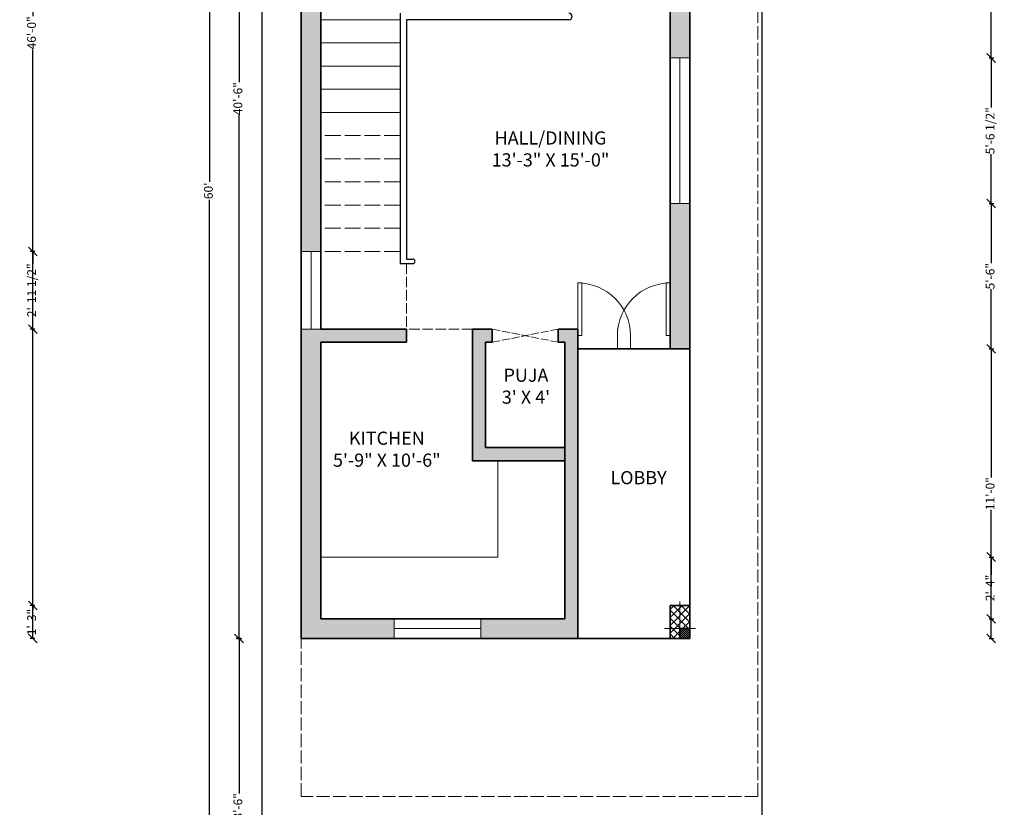
# Model space of a CAD drawing. Units: inches. Extents: x 2349 to 2798, y 397 to 1271.
# Tile 2 of 3: x 2349 to 2798, y 584 to 943. Entities that reach past the tile are written whole.
import ezdxf

# ---------------------------------------------------------------- set-up
doc = ezdxf.new("R2010")
doc.units = ezdxf.units.IN
doc.linetypes.add('ACAD_ISO02W100', pattern=[15, 12, -3])
for name, color, linetype, lineweight in [('A-ANNO-DIMS', 2, 'Continuous', 18), ('A-AREA-IDEN', 7, 'Continuous', 18), ('A-COLS', 1, 'Continuous', 35), ('A-COLS-CNTR', 253, 'Continuous', 13), ('A-COLS-PATT', 8, 'Continuous', 13), ('A-DOOR', 4, 'Continuous', 18), ('A-FLOR-FIXT', 30, 'Continuous', 18), ('A-FLOR-HRAL', 132, 'Continuous', 25), ('A-FLOR-OVHD', 253, 'ACAD_ISO02W100', 13), ('A-FLOR-STRS', 8, 'Continuous', 18), ('A-FLOR-STRS-OVHD', 8, 'ACAD_ISO02W100', 13), ('A-GLAZ', 4, 'Continuous', 18), ('A-WALL', 7, 'Continuous', 35), ('A-WALL-OVHD', 8, 'ACAD_ISO02W100', 13), ('A-WALL-PATT', 8, 'Continuous', 13), ('C-PROP', 7, 'Continuous', 25)]:
    doc.layers.add(name, color=color, linetype=linetype, lineweight=lineweight)
doc.styles.get("Standard").update_dxf_attribs({"font": 'arial.ttf'})
doc.dimstyles.new('ISO-25', dxfattribs={"dimtxt": 4, "dimasz": 4, "dimexe": 1.25, "dimexo": 1, "dimtad": 0, "dimdec": 1, "dimlunit": 3, "dimtxsty": 'Standard', "dimblk": 'OBLIQUE', "dimcen": 2.5, "dimclrd": 1, "dimclrt": 3, "dimadec": 0, "dimazin": 0, "dimtfac": 1, "dimtdec": 1, "dimtmove": 0, "dimatfit": 3, "dimfxl": 1, "dimfxlon": 1, "dimarcsym": 0})

# ---------------------------------------------------------------- blocks, each defined once
blk = doc.blocks.new('_Oblique')
at = {"color": 0, "linetype": 'ByBlock', "lineweight": -2}
blk.add_line((-0.5, -0.5), (0.5, 0.5), dxfattribs=at)
blk = doc.blocks.new('*D8')
at = {"layer": 'A-ANNO-DIMS', "color": 0, "lineweight": -2, "transparency": 16777216}
for p, q in [((2450.39, 1152.52), (2448.14, 1152.52)), ((2449.39, 1152.52), (2449.39, 914.09)), ((2449.39, 660.52), (2449.39, 898.94)), ((2448.39, 660.52), (2450.64, 660.52))]:
    blk.add_line(p, q, dxfattribs=at)
at = {"layer": 'Defpoints', "color": 0, "transparency": 16777216}
for p in [(2459.73, 1152.52), (2435.42, 660.52), (2449.39, 660.52)]:
    blk.add_point(p, dxfattribs=at)
at = {"layer": 'A-ANNO-DIMS', "color": 0, "lineweight": -2, "transparency": 16777216, "xscale": 4, "yscale": 4, "zscale": 4}
for p, rotation in [((2449.39, 1152.52), 90), ((2449.39, 660.52), 270)]:
    blk.add_blockref('_Oblique', p, dxfattribs=dict(at, rotation=rotation))
at = {"layer": 'A-ANNO-DIMS', "color": 0, "transparency": 16777216, "insert": (2449.39, 906.52), "char_height": 4, "attachment_point": 5, "rotation": 90}
blk.add_mtext('40\'-6"', dxfattribs=at)
blk = doc.blocks.new('*D9')
at = {"layer": 'A-ANNO-DIMS', "color": 0, "lineweight": -2, "transparency": 16777216}
for p, q in [((2450.39, 660.52), (2448.14, 660.52)), ((2449.39, 660.52), (2449.39, 589.82)), ((2449.39, 504.52), (2449.39, 575.21)), ((2450.39, 504.52), (2448.14, 504.52))]:
    blk.add_line(p, q, dxfattribs=at)
at = {"layer": 'Defpoints', "color": 0, "transparency": 16777216}
for p in [(2459.73, 660.52), (2449.39, 504.52), (2459.73, 504.52)]:
    blk.add_point(p, dxfattribs=at)
at = {"layer": 'A-ANNO-DIMS', "color": 0, "lineweight": -2, "transparency": 16777216, "xscale": 4, "yscale": 4, "zscale": 4}
for p, rotation in [((2449.39, 660.52), 90), ((2449.39, 504.52), 270)]:
    blk.add_blockref('_Oblique', p, dxfattribs=dict(at, rotation=rotation))
at = {"layer": 'A-ANNO-DIMS', "color": 0, "transparency": 16777216, "insert": (2449.39, 582.52), "char_height": 4, "attachment_point": 5, "rotation": 90}
blk.add_mtext('13\'-6"', dxfattribs=at)
blk = doc.blocks.new('*D10')
at = {"layer": 'A-ANNO-DIMS', "color": 0, "lineweight": -2, "transparency": 16777216}
for p, q in [((2436.96, 1224.52), (2434.71, 1224.52)), ((2435.96, 1224.52), (2435.96, 868.55)), ((2435.96, 504.52), (2435.96, 860.49)), ((2436.96, 504.52), (2434.71, 504.52))]:
    blk.add_line(p, q, dxfattribs=at)
at = {"layer": 'Defpoints', "color": 0, "transparency": 16777216}
for p in [(2459.73, 1224.52), (2435.96, 504.52), (2459.73, 504.52)]:
    blk.add_point(p, dxfattribs=at)
at = {"layer": 'A-ANNO-DIMS', "color": 0, "lineweight": -2, "transparency": 16777216, "xscale": 4, "yscale": 4, "zscale": 4}
for p, rotation in [((2435.96, 1224.52), 90), ((2435.96, 504.52), 270)]:
    blk.add_blockref('_Oblique', p, dxfattribs=dict(at, rotation=rotation))
at = {"layer": 'A-ANNO-DIMS', "color": 0, "transparency": 16777216, "insert": (2435.96, 864.52), "char_height": 4, "attachment_point": 5, "rotation": 90}
blk.add_mtext("60'", dxfattribs=at)
blk = doc.blocks.new('*U16')
for p, q in [((0, 0), (0, -6)), ((24, 0), (24, -6))]:
    blk.add_line(p, q)
blk.add_lwpolyline([(0, 0), (0, 24), (1.75, 24), (1.75, 0)], close=True)
blk.add_arc((0, 0), 24, 0, 90)
blk = doc.blocks.new('*U15')
for p, q in [((-24, 0), (-24, -6)), ((0, 0), (0, -6))]:
    blk.add_line(p, q)
blk.add_lwpolyline([(0, 0), (0, 24), (-1.75, 24), (-1.75, 0)], close=True)
blk.add_arc((0, 0), 24, 90, 180)
blk = doc.blocks.new('*D19')
at = {"layer": 'A-ANNO-DIMS', "color": 0, "lineweight": -2, "transparency": 16777216}
for p, q in [((2356.46, 1212.52), (2354.21, 1212.52)), ((2356.46, 660.52), (2354.21, 660.52))]:
    blk.add_line(p, q, dxfattribs=at)
at = {"layer": 'A-ANNO-DIMS', "color": 1, "lineweight": -2, "transparency": 16777216}
for p, q in [((2355.46, 1212.52), (2355.46, 944.09)), ((2355.46, 660.52), (2355.46, 928.94))]:
    blk.add_line(p, q, dxfattribs=at)
at = {"layer": 'Defpoints', "color": 0, "transparency": 16777216}
for p in [(2355.46, 1212.52), (2477.73, 1212.52), (2477.73, 660.52)]:
    blk.add_point(p, dxfattribs=at)
at = {"layer": 'A-ANNO-DIMS', "color": 1, "lineweight": -2, "transparency": 16777216, "xscale": 4, "yscale": 4, "zscale": 4}
for p, rotation in [((2355.46, 1212.52), 90), ((2355.46, 660.52), 270)]:
    blk.add_blockref('_Oblique', p, dxfattribs=dict(at, rotation=rotation))
at = {"layer": 'A-ANNO-DIMS', "color": 3, "transparency": 16777216, "insert": (2355.46, 936.52), "char_height": 4, "attachment_point": 5, "rotation": 90}
blk.add_mtext('46\'-0"', dxfattribs=at)
blk = doc.blocks.new('*D20')
at = {"layer": 'A-ANNO-DIMS', "color": 0, "lineweight": -2, "transparency": 16777216}
for p, q in [((2790.99, 792.52), (2793.24, 792.52)), ((2790.99, 660.52), (2793.24, 660.52))]:
    blk.add_line(p, q, dxfattribs=at)
at = {"layer": 'A-ANNO-DIMS', "color": 1, "lineweight": -2, "transparency": 16777216}
for p, q in [((2791.99, 792.52), (2791.99, 733.82)), ((2791.99, 660.52), (2791.99, 719.21))]:
    blk.add_line(p, q, dxfattribs=at)
at = {"layer": 'Defpoints', "color": 0, "transparency": 16777216}
for p in [(2654.73, 792.52), (2791.99, 792.52), (2654.73, 660.52)]:
    blk.add_point(p, dxfattribs=at)
at = {"layer": 'A-ANNO-DIMS', "color": 1, "lineweight": -2, "transparency": 16777216, "xscale": 4, "yscale": 4, "zscale": 4}
for p, rotation in [((2791.99, 792.52), 90), ((2791.99, 660.52), 270)]:
    blk.add_blockref('_Oblique', p, dxfattribs=dict(at, rotation=rotation))
at = {"layer": 'A-ANNO-DIMS', "color": 3, "transparency": 16777216, "insert": (2791.99, 726.52), "char_height": 4, "attachment_point": 5, "rotation": 90}
blk.add_mtext('11\'-0"', dxfattribs=at)
blk = doc.blocks.new('*D21')
at = {"layer": 'A-ANNO-DIMS', "color": 0, "lineweight": -2, "transparency": 16777216}
for p, q in [((2790.99, 858.74), (2793.24, 858.74)), ((2790.99, 792.52), (2793.24, 792.52))]:
    blk.add_line(p, q, dxfattribs=at)
at = {"layer": 'A-ANNO-DIMS', "color": 1, "lineweight": -2, "transparency": 16777216}
for p, q in [((2791.99, 858.74), (2791.99, 831.57)), ((2791.99, 792.52), (2791.99, 819.69))]:
    blk.add_line(p, q, dxfattribs=at)
at = {"layer": 'Defpoints', "color": 0, "transparency": 16777216}
for p in [(2654.73, 858.74), (2791.99, 858.74), (2654.73, 792.52)]:
    blk.add_point(p, dxfattribs=at)
at = {"layer": 'A-ANNO-DIMS', "color": 1, "lineweight": -2, "transparency": 16777216, "xscale": 4, "yscale": 4, "zscale": 4}
for p, rotation in [((2791.99, 858.74), 90), ((2791.99, 792.52), 270)]:
    blk.add_blockref('_Oblique', p, dxfattribs=dict(at, rotation=rotation))
at = {"layer": 'A-ANNO-DIMS', "color": 3, "transparency": 16777216, "insert": (2791.99, 825.63), "char_height": 4, "attachment_point": 5, "rotation": 90}
blk.add_mtext('5\'-6"', dxfattribs=at)
blk = doc.blocks.new('*D22')
at = {"layer": 'A-ANNO-DIMS', "color": 0, "lineweight": -2, "transparency": 16777216}
for p, q in [((2790.99, 925.07), (2793.24, 925.07)), ((2790.99, 858.74), (2793.24, 858.74))]:
    blk.add_line(p, q, dxfattribs=at)
at = {"layer": 'A-ANNO-DIMS', "color": 1, "lineweight": -2, "transparency": 16777216}
for p, q in [((2791.99, 925.07), (2791.99, 902.51)), ((2791.99, 858.74), (2791.99, 881.3))]:
    blk.add_line(p, q, dxfattribs=at)
at = {"layer": 'Defpoints', "color": 0, "transparency": 16777216}
for p in [(2654.73, 925.07), (2791.99, 925.07), (2654.73, 858.74)]:
    blk.add_point(p, dxfattribs=at)
at = {"layer": 'A-ANNO-DIMS', "color": 1, "lineweight": -2, "transparency": 16777216, "xscale": 4, "yscale": 4, "zscale": 4}
for p, rotation in [((2791.99, 925.07), 90), ((2791.99, 858.74), 270)]:
    blk.add_blockref('_Oblique', p, dxfattribs=dict(at, rotation=rotation))
at = {"layer": 'A-ANNO-DIMS', "color": 3, "transparency": 16777216, "insert": (2791.99, 891.9), "char_height": 4, "attachment_point": 5, "rotation": 90}
blk.add_mtext('5\'-6 1/2"', dxfattribs=at)
blk = doc.blocks.new('*D23')
at = {"layer": 'A-ANNO-DIMS', "color": 0, "lineweight": -2, "transparency": 16777216}
for p, q in [((2790.99, 1010.67), (2793.24, 1010.67)), ((2790.99, 925.07), (2793.24, 925.07))]:
    blk.add_line(p, q, dxfattribs=at)
at = {"layer": 'A-ANNO-DIMS', "color": 1, "lineweight": -2, "transparency": 16777216}
for p, q in [((2791.99, 1010.67), (2791.99, 978.45)), ((2791.99, 925.07), (2791.99, 957.28))]:
    blk.add_line(p, q, dxfattribs=at)
at = {"layer": 'Defpoints', "color": 0, "transparency": 16777216}
for p in [(2654.73, 1010.67), (2791.99, 1010.67), (2654.73, 925.07)]:
    blk.add_point(p, dxfattribs=at)
at = {"layer": 'A-ANNO-DIMS', "color": 1, "lineweight": -2, "transparency": 16777216, "xscale": 4, "yscale": 4, "zscale": 4}
for p, rotation in [((2791.99, 1010.67), 90), ((2791.99, 925.07), 270)]:
    blk.add_blockref('_Oblique', p, dxfattribs=dict(at, rotation=rotation))
at = {"layer": 'A-ANNO-DIMS', "color": 3, "transparency": 16777216, "insert": (2791.99, 967.87), "char_height": 4, "attachment_point": 5, "rotation": 90}
blk.add_mtext('7\'-1 1/2"', dxfattribs=at)
blk = doc.blocks.new('*D28')
at = {"layer": 'A-ANNO-DIMS', "color": 0, "lineweight": -2, "transparency": 16777216}
for p, q in [((2603.73, 403.67), (2603.73, 401.42)), ((2654.73, 403.67), (2654.73, 401.42))]:
    blk.add_line(p, q, dxfattribs=at)
at = {"layer": 'A-ANNO-DIMS', "color": 1, "lineweight": -2, "transparency": 16777216}
for p, q in [((2603.73, 402.67), (2623.21, 402.67)), ((2654.73, 402.67), (2635.25, 402.67))]:
    blk.add_line(p, q, dxfattribs=at)
at = {"layer": 'Defpoints', "color": 0, "transparency": 16777216}
for p in [(2603.73, 660.52), (2654.73, 660.52), (2654.73, 402.67)]:
    blk.add_point(p, dxfattribs=at)
at = {"layer": 'A-ANNO-DIMS', "color": 1, "lineweight": -2, "transparency": 16777216, "xscale": 4, "yscale": 4, "zscale": 4, "rotation": 180}
blk.add_blockref('_Oblique', (2603.73, 402.67), dxfattribs=at)
at = {"layer": 'A-ANNO-DIMS', "color": 1, "lineweight": -2, "transparency": 16777216, "xscale": 4, "yscale": 4, "zscale": 4}
blk.add_blockref('_Oblique', (2654.73, 402.67), dxfattribs=at)
at = {"layer": 'A-ANNO-DIMS', "color": 3, "transparency": 16777216, "insert": (2629.23, 402.67), "char_height": 4, "attachment_point": 5}
blk.add_mtext('4\'-3"', dxfattribs=at)
blk = doc.blocks.new('*D29')
at = {"layer": 'A-ANNO-DIMS', "color": 0, "lineweight": -2, "transparency": 16777216}
for p, q in [((2477.73, 403.67), (2477.73, 401.42)), ((2520.04, 403.67), (2520.04, 401.42))]:
    blk.add_line(p, q, dxfattribs=at)
at = {"layer": 'A-ANNO-DIMS', "color": 1, "lineweight": -2, "transparency": 16777216}
for p, q in [((2477.73, 402.67), (2488.28, 402.67)), ((2520.04, 402.67), (2509.48, 402.67))]:
    blk.add_line(p, q, dxfattribs=at)
at = {"layer": 'Defpoints', "color": 0, "transparency": 16777216}
for p in [(2477.73, 660.52), (2520.04, 660.52), (2520.04, 402.67)]:
    blk.add_point(p, dxfattribs=at)
at = {"layer": 'A-ANNO-DIMS', "color": 1, "lineweight": -2, "transparency": 16777216, "xscale": 4, "yscale": 4, "zscale": 4, "rotation": 180}
blk.add_blockref('_Oblique', (2477.73, 402.67), dxfattribs=at)
at = {"layer": 'A-ANNO-DIMS', "color": 1, "lineweight": -2, "transparency": 16777216, "xscale": 4, "yscale": 4, "zscale": 4}
blk.add_blockref('_Oblique', (2520.04, 402.67), dxfattribs=at)
at = {"layer": 'A-ANNO-DIMS', "color": 3, "transparency": 16777216, "insert": (2498.88, 402.67), "char_height": 4, "attachment_point": 5}
blk.add_mtext('3\'-6 1/2"', dxfattribs=at)
blk = doc.blocks.new('*D30')
at = {"layer": 'A-ANNO-DIMS', "color": 0, "lineweight": -2, "transparency": 16777216}
for p, q in [((2520.04, 403.67), (2520.04, 401.42)), ((2559.59, 403.67), (2559.59, 401.42))]:
    blk.add_line(p, q, dxfattribs=at)
at = {"layer": 'A-ANNO-DIMS', "color": 1, "lineweight": -2, "transparency": 16777216}
for p, q in [((2520.04, 402.67), (2529.21, 402.67)), ((2559.59, 402.67), (2550.42, 402.67))]:
    blk.add_line(p, q, dxfattribs=at)
at = {"layer": 'Defpoints', "color": 0, "transparency": 16777216}
for p in [(2520.04, 660.52), (2559.59, 660.52), (2559.59, 402.67)]:
    blk.add_point(p, dxfattribs=at)
at = {"layer": 'A-ANNO-DIMS', "color": 1, "lineweight": -2, "transparency": 16777216, "xscale": 4, "yscale": 4, "zscale": 4, "rotation": 180}
blk.add_blockref('_Oblique', (2520.04, 402.67), dxfattribs=at)
at = {"layer": 'A-ANNO-DIMS', "color": 1, "lineweight": -2, "transparency": 16777216, "xscale": 4, "yscale": 4, "zscale": 4}
blk.add_blockref('_Oblique', (2559.59, 402.67), dxfattribs=at)
at = {"layer": 'A-ANNO-DIMS', "color": 3, "transparency": 16777216, "insert": (2539.81, 402.67), "char_height": 4, "attachment_point": 5}
blk.add_mtext('3\'-3 1/2"', dxfattribs=at)
blk = doc.blocks.new('*D31')
at = {"layer": 'A-ANNO-DIMS', "color": 0, "lineweight": -2, "transparency": 16777216}
for p, q in [((2603.73, 403.67), (2603.73, 401.42)), ((2645.73, 403.67), (2645.73, 401.42))]:
    blk.add_line(p, q, dxfattribs=at)
at = {"layer": 'A-ANNO-DIMS', "color": 1, "lineweight": -2, "transparency": 16777216}
for p, q in [((2603.73, 402.67), (2618.79, 402.67)), ((2645.73, 402.67), (2630.67, 402.67))]:
    blk.add_line(p, q, dxfattribs=at)
at = {"layer": 'Defpoints', "color": 0, "transparency": 16777216}
for p in [(2603.73, 792.52), (2645.73, 792.52), (2645.73, 402.67)]:
    blk.add_point(p, dxfattribs=at)
at = {"layer": 'A-ANNO-DIMS', "color": 1, "lineweight": -2, "transparency": 16777216, "xscale": 4, "yscale": 4, "zscale": 4, "rotation": 180}
blk.add_blockref('_Oblique', (2603.73, 402.67), dxfattribs=at)
at = {"layer": 'A-ANNO-DIMS', "color": 1, "lineweight": -2, "transparency": 16777216, "xscale": 4, "yscale": 4, "zscale": 4}
blk.add_blockref('_Oblique', (2645.73, 402.67), dxfattribs=at)
at = {"layer": 'A-ANNO-DIMS', "color": 3, "transparency": 16777216, "insert": (2624.73, 402.67), "char_height": 4, "attachment_point": 5}
blk.add_mtext('3\'-6"', dxfattribs=at)
blk = doc.blocks.new('*D32')
at = {"layer": 'A-ANNO-DIMS', "color": 0, "lineweight": -2, "transparency": 16777216}
for p, q in [((2606.73, 403.67), (2606.73, 401.42)), ((2642.73, 403.67), (2642.73, 401.42))]:
    blk.add_line(p, q, dxfattribs=at)
at = {"layer": 'A-ANNO-DIMS', "color": 1, "lineweight": -2, "transparency": 16777216}
for p, q in [((2606.73, 402.67), (2618.79, 402.67)), ((2642.73, 402.67), (2630.67, 402.67))]:
    blk.add_line(p, q, dxfattribs=at)
at = {"layer": 'Defpoints', "color": 0, "transparency": 16777216}
for p in [(2606.73, 981.52), (2642.73, 981.52), (2642.73, 402.67)]:
    blk.add_point(p, dxfattribs=at)
at = {"layer": 'A-ANNO-DIMS', "color": 1, "lineweight": -2, "transparency": 16777216, "xscale": 4, "yscale": 4, "zscale": 4, "rotation": 180}
blk.add_blockref('_Oblique', (2606.73, 402.67), dxfattribs=at)
at = {"layer": 'A-ANNO-DIMS', "color": 1, "lineweight": -2, "transparency": 16777216, "xscale": 4, "yscale": 4, "zscale": 4}
blk.add_blockref('_Oblique', (2642.73, 402.67), dxfattribs=at)
at = {"layer": 'A-ANNO-DIMS', "color": 3, "transparency": 16777216, "insert": (2624.73, 402.67), "char_height": 4, "attachment_point": 5}
blk.add_mtext('3\'-0"', dxfattribs=at)
blk = doc.blocks.new('*D33')
at = {"layer": 'A-ANNO-DIMS', "color": 0, "lineweight": -2, "transparency": 16777216}
for p, q in [((2556.73, 403.67), (2556.73, 401.42)), ((2588.73, 403.67), (2588.73, 401.42))]:
    blk.add_line(p, q, dxfattribs=at)
at = {"layer": 'A-ANNO-DIMS', "color": 1, "lineweight": -2, "transparency": 16777216}
for p, q in [((2556.73, 402.67), (2566.76, 402.67)), ((2588.73, 402.67), (2578.71, 402.67))]:
    blk.add_line(p, q, dxfattribs=at)
at = {"layer": 'Defpoints', "color": 0, "transparency": 16777216}
for p in [(2556.73, 1143.52), (2588.73, 1143.52), (2588.73, 402.67)]:
    blk.add_point(p, dxfattribs=at)
at = {"layer": 'A-ANNO-DIMS', "color": 1, "lineweight": -2, "transparency": 16777216, "xscale": 4, "yscale": 4, "zscale": 4, "rotation": 180}
blk.add_blockref('_Oblique', (2556.73, 402.67), dxfattribs=at)
at = {"layer": 'A-ANNO-DIMS', "color": 1, "lineweight": -2, "transparency": 16777216, "xscale": 4, "yscale": 4, "zscale": 4}
blk.add_blockref('_Oblique', (2588.73, 402.67), dxfattribs=at)
at = {"layer": 'A-ANNO-DIMS', "color": 3, "transparency": 16777216, "insert": (2572.73, 402.67), "char_height": 4, "attachment_point": 5}
blk.add_mtext('2\'-8"', dxfattribs=at)
blk = doc.blocks.new('*D38')
at = {"layer": 'A-ANNO-DIMS', "color": 0, "lineweight": -2, "transparency": 16777216}
for p, q in [((2356.46, 836.92), (2354.21, 836.92)), ((2356.46, 801.52), (2354.21, 801.52))]:
    blk.add_line(p, q, dxfattribs=at)
at = {"layer": 'A-ANNO-DIMS', "color": 1, "lineweight": -2, "transparency": 16777216}
for p, q in [((2355.46, 836.92), (2355.46, 831.41)), ((2355.46, 801.52), (2355.46, 807.03))]:
    blk.add_line(p, q, dxfattribs=at)
at = {"layer": 'Defpoints', "color": 0, "transparency": 16777216}
for p in [(2355.46, 836.92), (2477.73, 836.92), (2477.73, 801.52)]:
    blk.add_point(p, dxfattribs=at)
at = {"layer": 'A-ANNO-DIMS', "color": 1, "lineweight": -2, "transparency": 16777216, "xscale": 4, "yscale": 4, "zscale": 4}
for p, rotation in [((2355.46, 836.92), 90), ((2355.46, 801.52), 270)]:
    blk.add_blockref('_Oblique', p, dxfattribs=dict(at, rotation=rotation))
at = {"layer": 'A-ANNO-DIMS', "color": 3, "transparency": 16777216, "insert": (2355.46, 819.22), "char_height": 4, "attachment_point": 5, "rotation": 90}
blk.add_mtext('2\'-11 1/2"', dxfattribs=at)
blk = doc.blocks.new('*D39')
at = {"layer": 'A-ANNO-DIMS', "color": 0, "lineweight": -2, "transparency": 16777216}
for p, q in [((2486.73, 403.67), (2486.73, 401.42)), ((2522.73, 403.67), (2522.73, 401.42))]:
    blk.add_line(p, q, dxfattribs=at)
at = {"layer": 'A-ANNO-DIMS', "color": 1, "lineweight": -2, "transparency": 16777216}
for p, q in [((2486.73, 402.67), (2498.79, 402.67)), ((2522.73, 402.67), (2510.67, 402.67))]:
    blk.add_line(p, q, dxfattribs=at)
at = {"layer": 'Defpoints', "color": 0, "transparency": 16777216}
for p in [(2486.73, 836.92), (2522.73, 836.92), (2522.73, 402.67)]:
    blk.add_point(p, dxfattribs=at)
at = {"layer": 'A-ANNO-DIMS', "color": 1, "lineweight": -2, "transparency": 16777216, "xscale": 4, "yscale": 4, "zscale": 4, "rotation": 180}
blk.add_blockref('_Oblique', (2486.73, 402.67), dxfattribs=at)
at = {"layer": 'A-ANNO-DIMS', "color": 1, "lineweight": -2, "transparency": 16777216, "xscale": 4, "yscale": 4, "zscale": 4}
blk.add_blockref('_Oblique', (2522.73, 402.67), dxfattribs=at)
at = {"layer": 'A-ANNO-DIMS', "color": 3, "transparency": 16777216, "insert": (2504.73, 402.67), "char_height": 4, "attachment_point": 5}
blk.add_mtext('3\'-0"', dxfattribs=at)
blk = doc.blocks.new('*D40')
at = {"layer": 'A-ANNO-DIMS', "color": 0, "lineweight": -2, "transparency": 16777216}
for p, q in [((2525.73, 403.67), (2525.73, 401.42)), ((2555.73, 403.67), (2555.73, 401.42))]:
    blk.add_line(p, q, dxfattribs=at)
at = {"layer": 'A-ANNO-DIMS', "color": 1, "lineweight": -2, "transparency": 16777216}
for p, q in [((2525.73, 402.67), (2534.76, 402.67)), ((2555.73, 402.67), (2546.71, 402.67))]:
    blk.add_line(p, q, dxfattribs=at)
at = {"layer": 'Defpoints', "color": 0, "transparency": 16777216}
for p in [(2555.73, 801.52), (2525.73, 795.52), (2555.73, 402.67)]:
    blk.add_point(p, dxfattribs=at)
at = {"layer": 'A-ANNO-DIMS', "color": 1, "lineweight": -2, "transparency": 16777216, "xscale": 4, "yscale": 4, "zscale": 4, "rotation": 180}
blk.add_blockref('_Oblique', (2525.73, 402.67), dxfattribs=at)
at = {"layer": 'A-ANNO-DIMS', "color": 1, "lineweight": -2, "transparency": 16777216, "xscale": 4, "yscale": 4, "zscale": 4}
blk.add_blockref('_Oblique', (2555.73, 402.67), dxfattribs=at)
at = {"layer": 'A-ANNO-DIMS', "color": 3, "transparency": 16777216, "insert": (2540.73, 402.67), "char_height": 4, "attachment_point": 5}
blk.add_mtext('2\'-6"', dxfattribs=at)
blk = doc.blocks.new('*D41')
at = {"layer": 'A-ANNO-DIMS', "color": 0, "lineweight": -2, "transparency": 16777216}
for p, q in [((2564.73, 1264.12), (2564.73, 1266.37)), ((2594.73, 1264.12), (2594.73, 1266.37))]:
    blk.add_line(p, q, dxfattribs=at)
at = {"layer": 'A-ANNO-DIMS', "color": 1, "lineweight": -2, "transparency": 16777216}
for p, q in [((2564.73, 1265.12), (2573.76, 1265.12)), ((2594.73, 1265.12), (2585.71, 1265.12))]:
    blk.add_line(p, q, dxfattribs=at)
at = {"layer": 'Defpoints', "color": 0, "transparency": 16777216}
for p in [(2594.73, 1265.12), (2564.73, 801.52), (2594.73, 801.52)]:
    blk.add_point(p, dxfattribs=at)
at = {"layer": 'A-ANNO-DIMS', "color": 1, "lineweight": -2, "transparency": 16777216, "xscale": 4, "yscale": 4, "zscale": 4, "rotation": 180}
blk.add_blockref('_Oblique', (2564.73, 1265.12), dxfattribs=at)
at = {"layer": 'A-ANNO-DIMS', "color": 1, "lineweight": -2, "transparency": 16777216, "xscale": 4, "yscale": 4, "zscale": 4}
blk.add_blockref('_Oblique', (2594.73, 1265.12), dxfattribs=at)
at = {"layer": 'A-ANNO-DIMS', "color": 3, "transparency": 16777216, "insert": (2579.73, 1265.12), "char_height": 4, "attachment_point": 5}
blk.add_mtext('2\'-6"', dxfattribs=at)
blk = doc.blocks.new('*D42')
at = {"layer": 'A-ANNO-DIMS', "color": 0, "lineweight": -2, "transparency": 16777216}
for p, q in [((2567.33, 1264.12), (2567.33, 1266.37)), ((2597.73, 1264.12), (2597.73, 1266.37))]:
    blk.add_line(p, q, dxfattribs=at)
at = {"layer": 'A-ANNO-DIMS', "color": 1, "lineweight": -2, "transparency": 16777216}
for p, q in [((2567.33, 1265.12), (2571.89, 1265.12)), ((2597.73, 1265.12), (2593.16, 1265.12))]:
    blk.add_line(p, q, dxfattribs=at)
at = {"layer": 'Defpoints', "color": 0, "transparency": 16777216}
for p in [(2567.33, 1265.12), (2567.33, 697.63), (2597.73, 669.52)]:
    blk.add_point(p, dxfattribs=at)
at = {"layer": 'A-ANNO-DIMS', "color": 1, "lineweight": -2, "transparency": 16777216, "xscale": 4, "yscale": 4, "zscale": 4, "rotation": 180}
blk.add_blockref('_Oblique', (2567.33, 1265.12), dxfattribs=at)
at = {"layer": 'A-ANNO-DIMS', "color": 1, "lineweight": -2, "transparency": 16777216, "xscale": 4, "yscale": 4, "zscale": 4}
blk.add_blockref('_Oblique', (2597.73, 1265.12), dxfattribs=at)
at = {"layer": 'A-ANNO-DIMS', "color": 3, "transparency": 16777216, "insert": (2582.53, 1265.12), "char_height": 4, "attachment_point": 5}
blk.add_mtext('2\'-6 1/2"', dxfattribs=at)
blk = doc.blocks.new('*D43')
at = {"layer": 'A-ANNO-DIMS', "color": 0, "lineweight": -2, "transparency": 16777216}
for p, q in [((2790.99, 697.63), (2793.24, 697.63)), ((2790.99, 669.52), (2793.24, 669.52))]:
    blk.add_line(p, q, dxfattribs=at)
at = {"layer": 'A-ANNO-DIMS', "color": 1, "lineweight": -2, "transparency": 16777216}
for p, q in [((2791.99, 697.63), (2791.99, 689.55)), ((2791.99, 669.52), (2791.99, 677.6))]:
    blk.add_line(p, q, dxfattribs=at)
at = {"layer": 'Defpoints', "color": 0, "transparency": 16777216}
for p in [(2486.73, 697.63), (2791.99, 697.63), (2486.73, 669.52)]:
    blk.add_point(p, dxfattribs=at)
at = {"layer": 'A-ANNO-DIMS', "color": 1, "lineweight": -2, "transparency": 16777216, "xscale": 4, "yscale": 4, "zscale": 4}
for p, rotation in [((2791.99, 697.63), 90), ((2791.99, 669.52), 270)]:
    blk.add_blockref('_Oblique', p, dxfattribs=dict(at, rotation=rotation))
at = {"layer": 'A-ANNO-DIMS', "color": 3, "transparency": 16777216, "insert": (2791.99, 683.57), "char_height": 4, "attachment_point": 5, "rotation": 90}
blk.add_mtext('2\'-4"', dxfattribs=at)
blk = doc.blocks.new('*D44')
at = {"layer": 'A-ANNO-DIMS', "color": 0, "lineweight": -2, "transparency": 16777216}
for p, q in [((2645.73, 1264.12), (2645.73, 1266.37)), ((2654.73, 1264.12), (2654.73, 1266.37))]:
    blk.add_line(p, q, dxfattribs=at)
at = {"layer": 'A-ANNO-DIMS', "color": 1, "lineweight": -2, "transparency": 16777216}
for p, q in [((2645.73, 1265.12), (2654.73, 1265.12)), ((2654.73, 1265.12), (2658.73, 1265.12))]:
    blk.add_line(p, q, dxfattribs=at)
at = {"layer": 'Defpoints', "color": 0, "transparency": 16777216}
for p in [(2654.73, 1265.12), (2645.73, 675.52), (2654.73, 675.52)]:
    blk.add_point(p, dxfattribs=at)
at = {"layer": 'A-ANNO-DIMS', "color": 1, "lineweight": -2, "transparency": 16777216, "xscale": 4, "yscale": 4, "zscale": 4, "rotation": 180}
blk.add_blockref('_Oblique', (2645.73, 1265.12), dxfattribs=at)
at = {"layer": 'A-ANNO-DIMS', "color": 1, "lineweight": -2, "transparency": 16777216, "xscale": 4, "yscale": 4, "zscale": 4}
blk.add_blockref('_Oblique', (2654.73, 1265.12), dxfattribs=at)
at = {"layer": 'A-ANNO-DIMS', "color": 3, "transparency": 16777216, "insert": (2664.67, 1265.12), "char_height": 4, "attachment_point": 5}
blk.add_mtext('0\'-9"', dxfattribs=at)
blk = doc.blocks.new('*D45')
at = {"layer": 'A-ANNO-DIMS', "color": 0, "lineweight": -2, "transparency": 16777216}
for p, q in [((2356.46, 675.52), (2354.21, 675.52)), ((2356.46, 660.52), (2354.21, 660.52))]:
    blk.add_line(p, q, dxfattribs=at)
at = {"layer": 'A-ANNO-DIMS', "color": 1, "lineweight": -2, "transparency": 16777216}
for p, q in [((2355.46, 675.52), (2355.46, 673.77)), ((2355.46, 660.52), (2355.46, 662.26))]:
    blk.add_line(p, q, dxfattribs=at)
at = {"layer": 'Defpoints', "color": 0, "transparency": 16777216}
for p in [(2355.46, 675.52), (2645.73, 675.52), (2645.73, 660.52)]:
    blk.add_point(p, dxfattribs=at)
at = {"layer": 'A-ANNO-DIMS', "color": 1, "lineweight": -2, "transparency": 16777216, "xscale": 4, "yscale": 4, "zscale": 4}
for p, rotation in [((2355.46, 675.52), 90), ((2355.46, 660.52), 270)]:
    blk.add_blockref('_Oblique', p, dxfattribs=dict(at, rotation=rotation))
at = {"layer": 'A-ANNO-DIMS', "color": 3, "transparency": 16777216, "insert": (2355.46, 668.02), "char_height": 4, "attachment_point": 5, "rotation": 90}
blk.add_mtext('1\'-3"', dxfattribs=at)
blk = doc.blocks.new('*D46')
at = {"layer": 'A-ANNO-DIMS', "color": 0, "lineweight": -2, "transparency": 16777216}
for p, q in [((2591.73, 403.67), (2591.73, 401.42)), ((2597.73, 403.67), (2597.73, 401.42))]:
    blk.add_line(p, q, dxfattribs=at)
at = {"layer": 'A-ANNO-DIMS', "color": 1, "lineweight": -2, "transparency": 16777216}
for p, q in [((2591.73, 402.67), (2597.73, 402.67)), ((2597.73, 402.67), (2601.73, 402.67))]:
    blk.add_line(p, q, dxfattribs=at)
at = {"layer": 'Defpoints', "color": 0, "transparency": 16777216}
for p in [(2591.73, 1206.52), (2597.73, 1206.52), (2597.73, 402.67)]:
    blk.add_point(p, dxfattribs=at)
at = {"layer": 'A-ANNO-DIMS', "color": 1, "lineweight": -2, "transparency": 16777216, "xscale": 4, "yscale": 4, "zscale": 4, "rotation": 180}
blk.add_blockref('_Oblique', (2591.73, 402.67), dxfattribs=at)
at = {"layer": 'A-ANNO-DIMS', "color": 1, "lineweight": -2, "transparency": 16777216, "xscale": 4, "yscale": 4, "zscale": 4}
blk.add_blockref('_Oblique', (2597.73, 402.67), dxfattribs=at)
at = {"layer": 'A-ANNO-DIMS', "color": 3, "transparency": 16777216, "insert": (2607.67, 402.67), "char_height": 4, "attachment_point": 5}
blk.add_mtext('0\'-6"', dxfattribs=at)
blk = doc.blocks.new('*D47')
at = {"layer": 'A-ANNO-DIMS', "color": 0, "lineweight": -2, "transparency": 16777216}
for p, q in [((2477.73, 403.67), (2477.73, 401.42)), ((2486.73, 403.67), (2486.73, 401.42))]:
    blk.add_line(p, q, dxfattribs=at)
at = {"layer": 'A-ANNO-DIMS', "color": 1, "lineweight": -2, "transparency": 16777216}
for p, q in [((2477.73, 402.67), (2486.73, 402.67)), ((2486.73, 402.67), (2490.73, 402.67))]:
    blk.add_line(p, q, dxfattribs=at)
at = {"layer": 'Defpoints', "color": 0, "transparency": 16777216}
for p in [(2477.73, 1212.52), (2486.73, 1206.52), (2486.73, 402.67)]:
    blk.add_point(p, dxfattribs=at)
at = {"layer": 'A-ANNO-DIMS', "color": 1, "lineweight": -2, "transparency": 16777216, "xscale": 4, "yscale": 4, "zscale": 4, "rotation": 180}
blk.add_blockref('_Oblique', (2477.73, 402.67), dxfattribs=at)
at = {"layer": 'A-ANNO-DIMS', "color": 1, "lineweight": -2, "transparency": 16777216, "xscale": 4, "yscale": 4, "zscale": 4}
blk.add_blockref('_Oblique', (2486.73, 402.67), dxfattribs=at)
at = {"layer": 'A-ANNO-DIMS', "color": 3, "transparency": 16777216, "insert": (2496.67, 402.67), "char_height": 4, "attachment_point": 5}
blk.add_mtext('0\'-9"', dxfattribs=at)
blk = doc.blocks.new('*D48')
at = {"layer": 'A-ANNO-DIMS', "color": 0, "lineweight": -2, "transparency": 16777216}
for p, q in [((2525.73, 403.67), (2525.73, 401.42)), ((2599.63, 403.67), (2599.63, 401.42))]:
    blk.add_line(p, q, dxfattribs=at)
at = {"layer": 'A-ANNO-DIMS', "color": 1, "lineweight": -2, "transparency": 16777216}
for p, q in [((2525.73, 402.67), (2556.73, 402.67)), ((2599.63, 402.67), (2568.63, 402.67))]:
    blk.add_line(p, q, dxfattribs=at)
at = {"layer": 'Defpoints', "color": 0, "transparency": 16777216}
for p in [(2525.73, 942.52), (2599.63, 942.52), (2599.63, 402.67)]:
    blk.add_point(p, dxfattribs=at)
at = {"layer": 'A-ANNO-DIMS', "color": 1, "lineweight": -2, "transparency": 16777216, "xscale": 4, "yscale": 4, "zscale": 4, "rotation": 180}
blk.add_blockref('_Oblique', (2525.73, 402.67), dxfattribs=at)
at = {"layer": 'A-ANNO-DIMS', "color": 1, "lineweight": -2, "transparency": 16777216, "xscale": 4, "yscale": 4, "zscale": 4}
blk.add_blockref('_Oblique', (2599.63, 402.67), dxfattribs=at)
at = {"layer": 'A-ANNO-DIMS', "color": 3, "transparency": 16777216, "insert": (2562.68, 402.67), "char_height": 4, "attachment_point": 5}
blk.add_mtext('6\'-2"', dxfattribs=at)

msp = doc.modelspace()

# ---------------------------------------------------------------- hatches: boundary and pattern name
at = {"layer": 'A-COLS-PATT'}
h = msp.add_hatch(dxfattribs=at)
h.set_pattern_fill('ANSI37', color=256, scale=0.8)
h.paths.add_polyline_path([(2654.73, 675.52), (2645.73, 675.52), (2645.73, 660.52), (2650.23, 660.52), (2650.23, 665.02), (2654.73, 665.02)])
h = msp.add_hatch(dxfattribs=at)
h.set_pattern_fill('ANSI31', color=256, scale=0.2)
h.paths.add_polyline_path([(2654.73, 665.02), (2650.23, 665.02), (2650.23, 660.52), (2654.73, 660.52)])
at = {"layer": 'A-WALL-PATT'}
h = msp.add_hatch(color=256, dxfattribs=at)
h.dxf.hatch_style = 1
h.paths.add_polyline_path([(2616.29, 1212.52), (2561.36, 1212.52), (2561.36, 1206.52), (2591.73, 1206.52), (2591.73, 1152.52), (2588.73, 1152.52), (2588.73, 1143.52), (2645.73, 1143.52), (2645.73, 1070.67), (2654.73, 1070.67), (2654.73, 1155.52), (2645.73, 1155.52), (2645.73, 1152.52), (2597.73, 1152.52), (2597.73, 1206.52), (2616.29, 1206.52)])
h.paths.add_polyline_path([(2654.73, 1212.52), (2637.4, 1212.52), (2637.4, 1206.52), (2645.73, 1206.52), (2645.73, 1183.52), (2654.73, 1183.52)], flags=17)
h.paths.add_polyline_path([(2520.04, 669.52), (2486.73, 669.52), (2486.73, 795.52), (2525.73, 795.52), (2525.73, 801.52), (2486.73, 801.52), (2477.73, 801.52), (2477.73, 660.52), (2520.04, 660.52)])
h.paths.add_polyline_path([(2486.73, 981.52), (2606.73, 981.52), (2606.73, 987.52), (2486.73, 987.52), (2486.73, 1143.52), (2556.73, 1143.52), (2556.73, 1152.52), (2486.73, 1152.52), (2486.73, 1206.52), (2534.27, 1206.52), (2534.27, 1212.52), (2477.73, 1212.52), (2477.73, 836.92), (2486.73, 836.92)])
h.paths.add_polyline_path([(2597.73, 747.52), (2561.73, 747.52), (2561.73, 795.52), (2564.73, 795.52), (2564.73, 801.52), (2555.73, 801.52), (2555.73, 741.52), (2597.73, 741.52)])
h.paths.add_polyline_path([(2654.73, 1010.67), (2645.73, 1010.67), (2645.73, 987.52), (2642.73, 987.52), (2642.73, 981.52), (2645.73, 981.52), (2645.73, 925.07), (2654.73, 925.07)])
h.paths.add_polyline_path([(2645.73, 858.74), (2645.73, 792.52), (2654.73, 792.52), (2654.73, 858.74)])
h.paths.add_polyline_path([(2603.73, 660.52), (2603.73, 801.52), (2594.73, 801.52), (2594.73, 795.52), (2597.73, 795.52), (2597.73, 669.52), (2559.59, 669.52), (2559.59, 660.52)])

# ---------------------------------------------------------------- linework, layer by layer
at = {"layer": 'A-COLS'}
for p, q in [((2645.73, 660.52), (2645.73, 675.52)), ((2645.73, 675.52), (2654.73, 675.52)), ((2654.73, 660.52), (2654.73, 675.52)), ((2650.23, 660.52), (2650.23, 665.02)), ((2650.23, 665.02), (2654.73, 665.02)), ((2654.73, 660.52), (2645.73, 660.52))]:
    msp.add_line(p, q, dxfattribs=at)
at = {"layer": 'A-COLS-CNTR'}
for p, q in [((2650.23, 665.02), (2650.23, 677.34)), ((2650.23, 665.02), (2643.15, 665.02)), ((2657.37, 665.02), (2654.73, 665.02))]:
    msp.add_line(p, q, dxfattribs=at)
at = {"layer": 'A-FLOR-FIXT'}
for p, q in [((2567.33, 741.52), (2567.33, 697.63)), ((2567.33, 697.63), (2486.73, 697.63))]:
    msp.add_line(p, q, dxfattribs=at)
at = {"layer": 'A-FLOR-HRAL'}
for p, q in [((2522.73, 945.52), (2522.73, 831.4)), ((2525.73, 942.52), (2525.73, 833.4)), ((2599.63, 942.52), (2525.73, 942.52)), ((2522.73, 831.4), (2528.61, 831.4)), ((2525.73, 833.4), (2528.61, 833.4))]:
    msp.add_line(p, q, dxfattribs=at)
for centre, radius in [((2599.63, 944.02), 1.5), ((2528.61, 832.4), 0.999)]:
    msp.add_arc(centre, radius, 270, 90, dxfattribs=at)
at = {"layer": 'A-FLOR-OVHD', "ltscale": 0.5}
for p, q in [((2685.73, 588.52), (2685.73, 1212.52)), ((2477.73, 588.52), (2477.73, 660.52)), ((2685.73, 588.52), (2477.73, 588.52))]:
    msp.add_line(p, q, dxfattribs=at)
at = {"layer": 'A-FLOR-STRS'}
for p, q in [((2522.73, 942.52), (2486.73, 942.52)), ((2522.73, 931.96), (2486.73, 931.96)), ((2522.73, 921.4), (2486.73, 921.4)), ((2522.73, 910.84), (2486.73, 910.84)), ((2522.73, 900.28), (2486.73, 900.28))]:
    msp.add_line(p, q, dxfattribs=at)
at = {"layer": 'A-FLOR-STRS-OVHD', "ltscale": 0.6}
for p, q in [((2522.73, 889.72), (2486.73, 889.72)), ((2522.73, 879.16), (2486.73, 879.16)), ((2522.73, 868.6), (2486.73, 868.6)), ((2522.73, 858.04), (2486.73, 858.04)), ((2522.73, 847.48), (2486.73, 847.48)), ((2522.73, 836.92), (2486.73, 836.92))]:
    msp.add_line(p, q, dxfattribs=at)
at = {"layer": 'A-FLOR-STRS-OVHD', "ltscale": 0.4}
msp.add_line((2525.73, 831.4), (2525.73, 801.52), dxfattribs=at)
at = {"layer": 'A-GLAZ'}
for p, q in [((2645.73, 925.07), (2654.73, 925.07)), ((2650.23, 858.74), (2650.23, 925.07)), ((2645.73, 858.74), (2654.73, 858.74)), ((2486.73, 836.92), (2477.73, 836.92)), ((2482.23, 836.92), (2482.23, 801.52)), ((2486.73, 801.52), (2477.73, 801.52)), ((2520.04, 669.52), (2520.04, 660.52)), ((2559.59, 669.52), (2559.59, 660.52)), ((2559.59, 665.02), (2520.04, 665.02))]:
    msp.add_line(p, q, dxfattribs=at)
at = {"layer": 'A-WALL'}
for p, q in [((2477.73, 1212.52), (2477.73, 660.52)), ((2654.73, 660.52), (2654.73, 1155.52)), ((2486.73, 981.52), (2486.73, 801.52)), ((2645.73, 792.52), (2645.73, 981.52)), ((2525.73, 801.52), (2486.73, 801.52)), ((2525.73, 801.52), (2525.73, 795.52)), ((2555.73, 741.52), (2555.73, 801.52)), ((2555.73, 801.52), (2564.73, 801.52)), ((2564.73, 795.52), (2564.73, 801.52)), ((2603.73, 801.52), (2594.73, 801.52)), ((2594.73, 795.52), (2594.73, 801.52)), ((2603.73, 801.52), (2603.73, 660.52)), ((2486.73, 795.52), (2486.73, 669.52)), ((2525.73, 795.52), (2486.73, 795.52)), ((2561.73, 747.52), (2561.73, 795.52)), ((2564.73, 795.52), (2561.73, 795.52)), ((2597.73, 795.52), (2594.73, 795.52)), ((2597.73, 795.52), (2597.73, 669.52)), ((2654.73, 792.52), (2603.73, 792.52)), ((2597.73, 747.52), (2561.73, 747.52)), ((2597.73, 741.52), (2555.73, 741.52)), ((2597.73, 669.52), (2486.73, 669.52)), ((2654.73, 660.52), (2477.73, 660.52))]:
    msp.add_line(p, q, dxfattribs=at)
at = {"layer": 'A-WALL-OVHD', "ltscale": 0.4}
msp.add_line((2555.73, 801.52), (2525.73, 801.52), dxfattribs=at)
at = {"layer": 'A-WALL-OVHD', "ltscale": 0.3}
for p, q in [((2564.73, 801.52), (2594.73, 795.52)), ((2594.73, 801.52), (2564.73, 795.52))]:
    msp.add_line(p, q, dxfattribs=at)
at = {"layer": 'C-PROP'}
for p, q in [((2459.73, 1224.52), (2459.73, 504.52)), ((2687.73, 504.52), (2687.73, 1224.52))]:
    msp.add_line(p, q, dxfattribs=at)

# ---------------------------------------------------------------- block references
at = {"layer": 'A-DOOR'}
for name, p in [('*U16', (2603.73, 798.52)), ('*U15', (2645.73, 798.52))]:
    msp.add_blockref(name, p, dxfattribs=at)

# ---------------------------------------------------------------- texts
at = {"layer": 'A-AREA-IDEN', "char_height": 6, "attachment_point": 1}
for s, width, insert in [('\\pxqc;HALL/DINING\\P13\'-3" X 15\'-0"', 82.6982, (2549.93, 891.61)), ("\\pxqc;PUJA\\P3' X 4'", 82.6982, (2538.75, 783.5)), ('\\pxqc;KITCHEN\\P5\'-9" X 10\'-6"', 65.6631, (2483.89, 754.79)), ('\\pxqc;LOBBY', 82.6982, (2590.02, 736.81))]:
    msp.add_mtext_dynamic_manual_height_columns(s, width=width, gutter_width=12.5, heights=[0], dxfattribs=dict(at, insert=insert))

# ---------------------------------------------------------------- dimensions: what is measured, and where the dimension line sits
at = {"layer": 'A-ANNO-DIMS'}
for base, p1, p2, picture, middle in [((2567.33, 1265.12), (2597.73, 669.52), (2567.33, 697.63), '*D42', (2582.53, 1265.12)), ((2594.73, 1265.12), (2564.73, 801.52), (2594.73, 801.52), '*D41', (2579.73, 1265.12)), ((2654.73, 1265.12), (2645.73, 675.52), (2654.73, 675.52), '*D44', (2664.67, 1265.12)), ((2486.73, 402.67), (2477.73, 1212.52), (2486.73, 1206.52), '*D47', (2496.67, 402.67)), ((2597.73, 402.67), (2591.73, 1206.52), (2597.73, 1206.52), '*D46', (2607.67, 402.67)), ((2588.73, 402.67), (2556.73, 1143.52), (2588.73, 1143.52), '*D33', (2572.73, 402.67)), ((2642.73, 402.67), (2606.73, 981.52), (2642.73, 981.52), '*D32', (2624.73, 402.67)), ((2599.63, 402.67), (2525.73, 942.52), (2599.63, 942.52), '*D48', (2562.68, 402.67)), ((2522.73, 402.67), (2486.73, 836.92), (2522.73, 836.92), '*D39', (2504.73, 402.67)), ((2555.73, 402.67), (2525.73, 795.52), (2555.73, 801.52), '*D40', (2540.73, 402.67)), ((2645.73, 402.67), (2603.73, 792.52), (2645.73, 792.52), '*D31', (2624.73, 402.67)), ((2520.04, 402.67), (2477.73, 660.52), (2520.04, 660.52), '*D29', (2498.88, 402.67)), ((2559.5941, 402.6665), (2520.0358, 660.5165), (2559.5941, 660.5165), '*D30', (2539.8149, 402.6665)), ((2654.73, 402.67), (2603.73, 660.52), (2654.73, 660.52), '*D28', (2629.23, 402.67))]:
    dim = msp.add_linear_dim(base=base, p1=p1, p2=p2, dimstyle='ISO-25', override={"dimdec": 1, "dimlfac": 1, "dimrnd": 0, "dimzin": 1, "dimdsep": 46, "dimlunit": 4, "dimfrac": 2}, dxfattribs=at)
    dim.commit()
    dim.dimension.update_dxf_attribs({"geometry": picture, "text_midpoint": middle})
for base, p1, p2, override, picture, middle in [((2435.96, 504.52), (2459.73, 1224.52), (2459.73, 504.52), {"dimclrd": 0, "dimclre": 0, "dimclrt": 0}, '*D10', (2435.96, 864.52)), ((2355.46, 1212.52), (2477.73, 660.52), (2477.73, 1212.52), {"dimdec": 1, "dimlfac": 1, "dimrnd": 0, "dimzin": 1, "dimdsep": 46, "dimlunit": 4, "dimfrac": 2}, '*D19', (2355.46, 936.52)), ((2791.99, 1010.67), (2654.73, 925.07), (2654.73, 1010.67), {"dimdec": 1, "dimlfac": 1, "dimrnd": 0, "dimzin": 1, "dimdsep": 46, "dimlunit": 4, "dimfrac": 2}, '*D23', (2791.99, 967.87)), ((2791.99, 925.07), (2654.73, 858.74), (2654.73, 925.07), {"dimdec": 1, "dimlfac": 1, "dimrnd": 0, "dimzin": 1, "dimdsep": 46, "dimlunit": 4, "dimfrac": 2}, '*D22', (2791.99, 891.9)), ((2791.99, 858.74), (2654.73, 792.52), (2654.73, 858.74), {"dimdec": 1, "dimlfac": 1, "dimrnd": 0, "dimzin": 1, "dimdsep": 46, "dimlunit": 4, "dimfrac": 2}, '*D21', (2791.99, 825.63)), ((2355.46, 836.92), (2477.73, 801.52), (2477.73, 836.92), {"dimdec": 1, "dimlfac": 1, "dimrnd": 0, "dimzin": 1, "dimdsep": 46, "dimlunit": 4, "dimfrac": 2}, '*D38', (2355.46, 819.22)), ((2791.99, 792.52), (2654.73, 660.52), (2654.73, 792.52), {"dimdec": 1, "dimlfac": 1, "dimrnd": 0, "dimzin": 1, "dimdsep": 46, "dimlunit": 4, "dimfrac": 2}, '*D20', (2791.99, 726.52)), ((2791.99, 697.63), (2486.73, 669.52), (2486.73, 697.63), {"dimdec": 1, "dimlfac": 1, "dimrnd": 0, "dimzin": 1, "dimdsep": 46, "dimlunit": 4, "dimfrac": 2}, '*D43', (2791.99, 683.57)), ((2355.46, 675.52), (2645.73, 660.52), (2645.73, 675.52), {"dimdec": 1, "dimlfac": 1, "dimrnd": 0, "dimzin": 1, "dimdsep": 46, "dimlunit": 4, "dimfrac": 2}, '*D45', (2355.46, 668.02))]:
    dim = msp.add_linear_dim(base=base, p1=p1, p2=p2, angle=90, dimstyle='ISO-25', override=override, dxfattribs=at)
    dim.commit()
    dim.dimension.update_dxf_attribs({"geometry": picture, "text_midpoint": middle})
for base, p1, p2, text, picture, middle in [((2449.39, 660.52), (2459.73, 1152.52), (2435.42, 660.52), '40\'-6"', '*D8', (2449.39, 906.52)), ((2449.39, 504.52), (2459.73, 660.52), (2459.73, 504.52), '13\'-6"', '*D9', (2449.39, 582.52))]:
    dim = msp.add_linear_dim(base=base, p1=p1, p2=p2, angle=90, text=text, dimstyle='ISO-25', override={"dimclrd": 0, "dimclre": 0, "dimclrt": 0, "dimtmove": 1}, dxfattribs=at)
    dim.commit()
    dim.dimension.update_dxf_attribs({"geometry": picture, "text_midpoint": middle})

doc.saveas('drawing.dxf')
